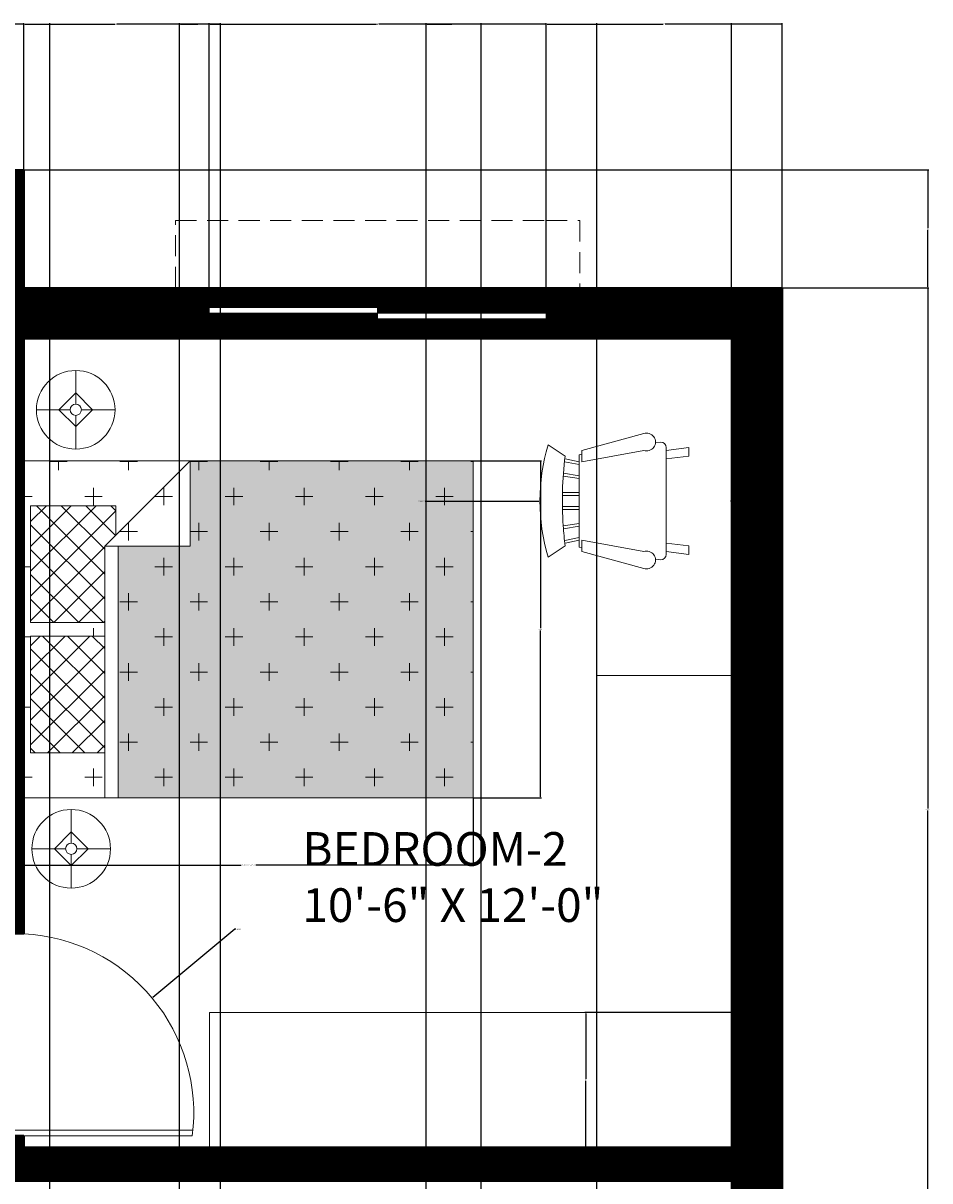
# Model space of a CAD drawing. Units: inches. Extents: x 557 to 1007, y 390 to 953.
# Tile 10 of 10: x 845 to 1007, y 747 to 953. Entities that reach past the tile are written whole.
import ezdxf

# ---------------------------------------------------------------- set-up
doc = ezdxf.new("R2010")
doc.units = ezdxf.units.IN
doc.header["$LTSCALE"] = 5
doc.header["$MEASUREMENT"] = 0
doc.linetypes.add('HIDDEN', pattern=[0.375, 0.25, -0.125])
for name, color, linetype, lineweight in [('A-ANNO-DIMS', 2, 'Continuous', 18), ('A-AREA-IDEN', 7, 'Continuous', 18), ('A-DOOR', 3, 'Continuous', 18), ('A-FLOR-CASE', 8, 'Continuous', 18), ('A-FURN', 8, 'Continuous', 18), ('A-FURN-PATT', 9, 'Continuous', 9), ('A-GLAZ', 4, 'Continuous', 18), ('A-GLAZ-OVHD', 8, 'HIDDEN', 13), ('A-WALL', 7, 'Continuous', 35), ('E-LITE', 2, 'Continuous', 13)]:
    doc.layers.add(name, color=color, linetype=linetype, lineweight=lineweight)
doc.layers.add('A-GLAZ-PATT', color=141, linetype='Continuous', lineweight=9, true_color=0xadddf7)
doc.layers.add('A-WALL-PATT', color=251, linetype='Continuous', lineweight=9, true_color=0x636466)
doc.styles.get("Standard").update_dxf_attribs({"font": 'arial.ttf'})
doc.dimstyles.get("Standard").update_dxf_attribs({"dimtxt": 0.18, "dimasz": 0.18, "dimexe": 0.18, "dimexo": 0.0625, "dimgap": 0.09, "dimtad": 0, "dimtih": 1, "dimtoh": 1, "dimdec": 4, "dimzin": 0, "dimdsep": 46, "dimtxsty": 'Standard', "dimcen": 0.09, "dimadec": 0, "dimazin": 0, "dimtfac": 1, "dimtdec": 4, "dimtofl": 0, "dimtmove": 0, "dimatfit": 3, "dimfxl": 1, "dimtolj": 1, "dimtzin": 0, "dimarcsym": 0})

# ---------------------------------------------------------------- blocks, each defined once
blk = doc.blocks.new('Chair - Rocking')
for p, q in [((-8, -4.5), (-10, -1.5)), ((8, -4.5), (10, -1.5)), ((-1.5, -4.05012), (-1.5, -7)), ((-1, -7), (-1, -4.05012)), ((1, -7), (1, -4.04655)), ((1.5, -4.05012), (1.5, -7)), ((-7.5, -4.5), (-7, -7)), ((-6.5, -7), (-7.02225, -4.43)), ((-4.5, -7), (-4.96674, -4.19951)), ((-4, -7), (-4.40532, -4.16272)), ((4, -7), (4.40187, -4.18694)), ((4.5, -7), (4.96761, -4.19437)), ((6.5, -7), (7, -4.4057)), ((7.5, -4.5), (7, -7)), ((-9, -7.5), (-12, -18.49999)), ((-7, -7.5), (-9, -7.5)), ((-9, -18.49999), (-7, -7.5)), ((-8.23428, -6.99939), (-8.3093, -7.47958)), ((-8.23041, -7), (8.23915, -7)), ((7, -7.5), (9, -7.5)), ((9, -18.49999), (7, -7.5)), ((8.31071, -7.48854), (8.23449, -7.00073)), ((9, -7.5), (12, -18.49999)), ((10.5, -21.49999), (10.3575, -20.58798)), ((-10.36644, -20.64523), (-10.5, -21.49999)), ((-9, -22.49999), (-9.5, -26.49999)), ((0, -22.49999), (-9.5, -22.49999)), ((-8, -26.49999), (-7.5, -22.49999)), ((0, -22.49999), (9.5, -22.49999)), ((8, -26.49999), (7.5, -22.49999)), ((9, -22.49999), (9.5, -26.49999)), ((-9.5, -26.49999), (-8, -26.49999)), ((9.5, -26.49999), (8, -26.49999))]:
    blk.add_line(p, q)
for centre, radius, start, end in [((0, -34.08333), 34.08333, 72.93847, 107.0615), ((0, -68.25004), 64.25, 82.84733, 93.92211), ((0, -68.25004), 64.25, 93.92211, 97.15267), ((-10.5, -18.99999), 1.58114, 161.5651, 18.43495), ((10.5, -18.99999), 1.58114, 161.5651, 18.43495), ((-9.5, -21.49999), 1, 180, 270), ((9.5, -21.49999), 1, 270, 0)]:
    blk.add_arc(centre, radius, start, end)
blk = doc.blocks.new('Lamp - Table')
for p, q in [((0, 7), (0, 1)), ((0, 3), (-3, 0)), ((3, 0), (0, 3)), ((-1, 0), (-7, 0)), ((-3, 0), (0, -3)), ((0, -3), (3, 0)), ((1, 0), (7, 0)), ((0, -1), (0, -7))]:
    blk.add_line(p, q)
for radius in [7, 1]:
    blk.add_circle((0, 0), radius)
blk = doc.blocks.new('BED-QUEEN-60x80-PLAN')
for p, q in [((0, 0), (0, 60)), ((0, 60), (80, 60)), ((29.6, 60), (14.4, 44.8)), ((29.6, 44.8), (29.6, 60)), ((80, 60), (80, 0)), ((1.2, 52), (16.4, 52)), ((1.2, 31.2), (1.2, 52)), ((16.4, 52), (16.4, 46.8)), ((14.4, 0), (14.4, 44.8)), ((14.4, 44.8), (29.6, 44.8)), ((16.8, 44.8), (16.8, 0)), ((14.4, 31.2), (1.2, 31.2)), ((1.2, 28.8), (14.4, 28.8)), ((1.2, 8), (1.2, 28.8)), ((14.4, 8), (1.2, 8)), ((80, 0), (0, 0))]:
    blk.add_line(p, q)
blk = doc.blocks.new('*D19')
at = {"layer": 'A-ANNO-DIMS', "color": 0, "lineweight": -2, "ltscale": 5, "transparency": 16777216}
for p, q in [((845.41, 815.04), (845.41, 802.92)), ((925.41, 815.04), (925.41, 802.92)), ((845.59, 803.1), (884.1, 803.1)), ((925.23, 803.1), (886.71, 803.1))]:
    blk.add_line(p, q, dxfattribs=at)
at = {"layer": 'A-ANNO-DIMS', "color": 0, "ltscale": 5, "transparency": 16777216}
for points in [[(845.59, 803.13), (845.59, 803.07), (845.41, 803.1)], [(925.23, 803.13), (925.23, 803.07), (925.41, 803.1)]]:
    blk.add_solid(points, dxfattribs=at)
at = {"layer": 'Defpoints', "color": 0, "ltscale": 5, "transparency": 16777216}
for p in [(845.41, 815.1), (925.41, 815.1), (925.41, 803.1)]:
    blk.add_point(p, dxfattribs=at)
at = {"layer": 'A-ANNO-DIMS', "color": 0, "ltscale": 5, "transparency": 16777216, "insert": (885.41, 803.1), "char_height": 0.18, "attachment_point": 5}
blk.add_mtext('\\A1;QUEEN BED 80 TYP.', dxfattribs=at)
blk = doc.blocks.new('*D20')
at = {"layer": 'A-ANNO-DIMS', "color": 0, "lineweight": -2, "ltscale": 5, "transparency": 16777216}
for p, q in [((925.47, 875.1), (937.59, 875.1)), ((937.41, 874.92), (937.41, 845.29)), ((937.41, 815.28), (937.41, 844.92)), ((925.47, 815.1), (937.59, 815.1))]:
    blk.add_line(p, q, dxfattribs=at)
at = {"layer": 'A-ANNO-DIMS', "color": 0, "ltscale": 5, "transparency": 16777216}
for points in [[(937.38, 874.92), (937.44, 874.92), (937.41, 875.1)], [(937.38, 815.28), (937.44, 815.28), (937.41, 815.1)]]:
    blk.add_solid(points, dxfattribs=at)
at = {"layer": 'Defpoints', "color": 0, "ltscale": 5, "transparency": 16777216}
for p in [(925.41, 875.1), (937.41, 875.1), (925.41, 815.1)]:
    blk.add_point(p, dxfattribs=at)
at = {"layer": 'A-ANNO-DIMS', "color": 0, "ltscale": 5, "transparency": 16777216, "insert": (937.41, 845.1), "char_height": 0.18, "attachment_point": 5}
blk.add_mtext('\\A1;60 TYP.', dxfattribs=at)
blk = doc.blocks.new('*D50')
at = {"layer": 'A-ANNO-DIMS', "color": 0, "lineweight": -2, "ltscale": 5, "transparency": 16777216}
for p, q in [((761.41, 926.97), (761.41, 953.03)), ((761.59, 952.85), (803.19, 952.85)), ((845.23, 952.85), (803.62, 952.85)), ((845.41, 926.97), (845.41, 953.03))]:
    blk.add_line(p, q, dxfattribs=at)
at = {"layer": 'A-ANNO-DIMS', "color": 0, "ltscale": 5, "transparency": 16777216}
for points in [[(761.59, 952.88), (761.59, 952.82), (761.41, 952.85)], [(845.23, 952.88), (845.23, 952.82), (845.41, 952.85)]]:
    blk.add_solid(points, dxfattribs=at)
at = {"layer": 'Defpoints', "color": 0, "ltscale": 5, "transparency": 16777216}
for p in [(845.41, 952.85), (761.41, 926.9), (845.41, 926.9)]:
    blk.add_point(p, dxfattribs=at)
at = {"layer": 'A-ANNO-DIMS', "color": 0, "ltscale": 5, "transparency": 16777216, "insert": (803.41, 952.85), "char_height": 0.18, "attachment_point": 5}
blk.add_mtext('\\A1;84', dxfattribs=at)
blk = doc.blocks.new('*D51')
at = {"layer": 'A-ANNO-DIMS', "color": 0, "lineweight": -2, "ltscale": 5, "transparency": 16777216}
for p, q in [((845.41, 905.97), (845.41, 953.03)), ((845.59, 952.85), (861.69, 952.85)), ((878.23, 952.85), (862.12, 952.85)), ((878.41, 905.97), (878.41, 953.03))]:
    blk.add_line(p, q, dxfattribs=at)
at = {"layer": 'A-ANNO-DIMS', "color": 0, "ltscale": 5, "transparency": 16777216}
for points in [[(845.59, 952.88), (845.59, 952.82), (845.41, 952.85)], [(878.23, 952.88), (878.23, 952.82), (878.41, 952.85)]]:
    blk.add_solid(points, dxfattribs=at)
at = {"layer": 'Defpoints', "color": 0, "ltscale": 5, "transparency": 16777216}
for p in [(878.41, 952.85), (845.41, 905.9), (878.41, 905.9)]:
    blk.add_point(p, dxfattribs=at)
at = {"layer": 'A-ANNO-DIMS', "color": 0, "ltscale": 5, "transparency": 16777216, "insert": (861.91, 952.85), "char_height": 0.18, "attachment_point": 5}
blk.add_mtext('\\A1;33', dxfattribs=at)
blk = doc.blocks.new('*D52')
at = {"layer": 'A-ANNO-DIMS', "color": 0, "lineweight": -2, "ltscale": 5, "transparency": 16777216}
for p, q in [((878.41, 905.97), (878.41, 953.03)), ((878.59, 952.85), (908.19, 952.85)), ((938.23, 952.85), (908.62, 952.85)), ((938.41, 905.97), (938.41, 953.03))]:
    blk.add_line(p, q, dxfattribs=at)
at = {"layer": 'A-ANNO-DIMS', "color": 0, "ltscale": 5, "transparency": 16777216}
for points in [[(878.59, 952.88), (878.59, 952.82), (878.41, 952.85)], [(938.23, 952.88), (938.23, 952.82), (938.41, 952.85)]]:
    blk.add_solid(points, dxfattribs=at)
at = {"layer": 'Defpoints', "color": 0, "ltscale": 5, "transparency": 16777216}
for p in [(938.41, 952.85), (878.41, 905.9), (938.41, 905.9)]:
    blk.add_point(p, dxfattribs=at)
at = {"layer": 'A-ANNO-DIMS', "color": 0, "ltscale": 5, "transparency": 16777216, "insert": (908.41, 952.85), "char_height": 0.18, "attachment_point": 5}
blk.add_mtext('\\A1;60', dxfattribs=at)
blk = doc.blocks.new('*D53')
at = {"layer": 'A-ANNO-DIMS', "color": 0, "lineweight": -2, "ltscale": 5, "transparency": 16777216}
for p, q in [((938.41, 905.97), (938.41, 953.03)), ((938.59, 952.85), (959.18, 952.85)), ((980.23, 952.85), (959.63, 952.85)), ((980.41, 905.97), (980.41, 953.03))]:
    blk.add_line(p, q, dxfattribs=at)
at = {"layer": 'A-ANNO-DIMS', "color": 0, "ltscale": 5, "transparency": 16777216}
for points in [[(938.59, 952.88), (938.59, 952.82), (938.41, 952.85)], [(980.23, 952.88), (980.23, 952.82), (980.41, 952.85)]]:
    blk.add_solid(points, dxfattribs=at)
at = {"layer": 'Defpoints', "color": 0, "ltscale": 5, "transparency": 16777216}
for p in [(980.41, 952.85), (938.41, 905.9), (980.41, 905.9)]:
    blk.add_point(p, dxfattribs=at)
at = {"layer": 'A-ANNO-DIMS', "color": 0, "ltscale": 5, "transparency": 16777216, "insert": (959.41, 952.85), "char_height": 0.18, "attachment_point": 5}
blk.add_mtext('\\A1;42', dxfattribs=at)
blk = doc.blocks.new('*D57')
at = {"layer": 'A-ANNO-DIMS', "color": 0, "lineweight": -2, "ltscale": 5, "transparency": 16777216}
for p, q in [((980.47, 905.9), (1006.54, 905.9)), ((1006.36, 905.72), (1006.36, 813.22)), ((1006.36, 720.36), (1006.36, 812.86)), ((980.47, 720.18), (1006.54, 720.18))]:
    blk.add_line(p, q, dxfattribs=at)
at = {"layer": 'A-ANNO-DIMS', "color": 0, "ltscale": 5, "transparency": 16777216}
for points in [[(1006.33, 905.72), (1006.39, 905.72), (1006.36, 905.9)], [(1006.33, 720.36), (1006.39, 720.36), (1006.36, 720.18)]]:
    blk.add_solid(points, dxfattribs=at)
at = {"layer": 'Defpoints', "color": 0, "ltscale": 5, "transparency": 16777216}
for p in [(980.41, 905.9), (1006.36, 905.9), (980.41, 720.18)]:
    blk.add_point(p, dxfattribs=at)
at = {"layer": 'A-ANNO-DIMS', "color": 0, "ltscale": 5, "transparency": 16777216, "insert": (1006.36, 813.04), "char_height": 0.18, "attachment_point": 5}
blk.add_mtext('\\A1;185.73', dxfattribs=at)
blk = doc.blocks.new('*D58')
at = {"layer": 'A-ANNO-DIMS', "color": 0, "lineweight": -2, "ltscale": 5, "transparency": 16777216}
for p, q in [((845.47, 926.9), (1006.54, 926.9)), ((1006.36, 926.72), (1006.36, 916.58)), ((1006.36, 906.08), (1006.36, 916.22)), ((980.47, 905.9), (1006.54, 905.9))]:
    blk.add_line(p, q, dxfattribs=at)
at = {"layer": 'A-ANNO-DIMS', "color": 0, "ltscale": 5, "transparency": 16777216}
for points in [[(1006.33, 926.72), (1006.39, 926.72), (1006.36, 926.9)], [(1006.33, 906.08), (1006.39, 906.08), (1006.36, 905.9)]]:
    blk.add_solid(points, dxfattribs=at)
at = {"layer": 'Defpoints', "color": 0, "ltscale": 5, "transparency": 16777216}
for p in [(845.41, 926.9), (1006.36, 926.9), (980.41, 905.9)]:
    blk.add_point(p, dxfattribs=at)
at = {"layer": 'A-ANNO-DIMS', "color": 0, "ltscale": 5, "transparency": 16777216, "insert": (1006.36, 916.4), "char_height": 0.18, "attachment_point": 5}
blk.add_mtext('\\A1;21', dxfattribs=at)
blk = doc.blocks.new('*D82')
at = {"layer": 'A-ANNO-DIMS', "color": 0, "lineweight": -2, "ltscale": 5, "transparency": 16777216}
for p, q in [((850.01, 665.94), (850.01, 953.03)), ((850.19, 952.85), (861.18, 952.85)), ((872.97, 952.85), (861.98, 952.85)), ((873.15, 661.94), (873.15, 953.03))]:
    blk.add_line(p, q, dxfattribs=at)
at = {"layer": 'A-ANNO-DIMS', "color": 0, "ltscale": 5, "transparency": 16777216}
for points in [[(850.19, 952.88), (850.19, 952.82), (850.01, 952.85)], [(872.97, 952.88), (872.97, 952.82), (873.15, 952.85)]]:
    blk.add_solid(points, dxfattribs=at)
at = {"layer": 'Defpoints', "color": 0, "ltscale": 5, "transparency": 16777216}
for p in [(873.15, 952.85), (850.01, 665.88), (873.15, 661.88)]:
    blk.add_point(p, dxfattribs=at)
at = {"layer": 'A-ANNO-DIMS', "color": 0, "ltscale": 5, "transparency": 16777216, "insert": (861.58, 952.85), "char_height": 0.18, "attachment_point": 5}
blk.add_mtext('\\A1;23.13', dxfattribs=at)
blk = doc.blocks.new('*D86')
at = {"layer": 'A-ANNO-DIMS', "color": 0, "lineweight": -2, "ltscale": 5, "transparency": 16777216}
for p, q in [((873.15, 661.94), (873.15, 953.03)), ((873.33, 952.85), (876.4, 952.85)), ((880.27, 952.85), (877.19, 952.85)), ((880.45, 663.9), (880.45, 953.03))]:
    blk.add_line(p, q, dxfattribs=at)
at = {"layer": 'A-ANNO-DIMS', "color": 0, "ltscale": 5, "transparency": 16777216}
for points in [[(873.33, 952.88), (873.33, 952.82), (873.15, 952.85)], [(880.27, 952.88), (880.27, 952.82), (880.45, 952.85)]]:
    blk.add_solid(points, dxfattribs=at)
at = {"layer": 'Defpoints', "color": 0, "ltscale": 5, "transparency": 16777216}
for p in [(880.45, 952.85), (880.45, 663.84), (873.15, 661.88)]:
    blk.add_point(p, dxfattribs=at)
at = {"layer": 'A-ANNO-DIMS', "color": 0, "ltscale": 5, "transparency": 16777216, "insert": (876.8, 952.85), "char_height": 0.18, "attachment_point": 5}
blk.add_mtext('\\A1;7.303', dxfattribs=at)
blk = doc.blocks.new('*D87')
at = {"layer": 'A-ANNO-DIMS', "color": 0, "lineweight": -2, "ltscale": 5, "transparency": 16777216}
for p, q in [((917.05, 663.9), (917.05, 953.03)), ((917.23, 952.85), (921.61, 952.85)), ((926.63, 952.85), (922.26, 952.85)), ((926.81, 662.58), (926.81, 953.03))]:
    blk.add_line(p, q, dxfattribs=at)
at = {"layer": 'A-ANNO-DIMS', "color": 0, "ltscale": 5, "transparency": 16777216}
for points in [[(917.23, 952.88), (917.23, 952.82), (917.05, 952.85)], [(926.63, 952.88), (926.63, 952.82), (926.81, 952.85)]]:
    blk.add_solid(points, dxfattribs=at)
at = {"layer": 'Defpoints', "color": 0, "ltscale": 5, "transparency": 16777216}
for p in [(926.81, 952.85), (917.05, 663.84), (926.81, 662.52)]:
    blk.add_point(p, dxfattribs=at)
at = {"layer": 'A-ANNO-DIMS', "color": 0, "ltscale": 5, "transparency": 16777216, "insert": (921.93, 952.85), "char_height": 0.18, "attachment_point": 5}
blk.add_mtext('\\A1;9.76', dxfattribs=at)
blk = doc.blocks.new('*D96')
at = {"layer": 'A-ANNO-DIMS', "color": 0, "lineweight": -2, "ltscale": 5, "transparency": 16777216}
for p, q in [((947.41, 536.97), (947.41, 953.03)), ((947.59, 952.85), (959.19, 952.85)), ((971.23, 952.85), (959.63, 952.85)), ((971.41, 512.97), (971.41, 953.03))]:
    blk.add_line(p, q, dxfattribs=at)
at = {"layer": 'A-ANNO-DIMS', "color": 0, "ltscale": 5, "transparency": 16777216}
for points in [[(947.59, 952.88), (947.59, 952.82), (947.41, 952.85)], [(971.23, 952.88), (971.23, 952.82), (971.41, 952.85)]]:
    blk.add_solid(points, dxfattribs=at)
at = {"layer": 'Defpoints', "color": 0, "ltscale": 5, "transparency": 16777216}
for p in [(971.41, 952.85), (947.41, 536.9), (971.41, 512.9)]:
    blk.add_point(p, dxfattribs=at)
at = {"layer": 'A-ANNO-DIMS', "color": 0, "ltscale": 5, "transparency": 16777216, "insert": (959.41, 952.85), "char_height": 0.18, "attachment_point": 5}
blk.add_mtext('\\A1;24', dxfattribs=at)
blk = doc.blocks.new('*D97')
at = {"layer": 'A-ANNO-DIMS', "color": 0, "lineweight": -2, "ltscale": 5, "transparency": 16777216}
for p, q in [((971.34, 776.9), (945.28, 776.9)), ((945.46, 776.72), (945.46, 765.08)), ((945.46, 753.08), (945.46, 764.72)), ((971.34, 752.9), (945.28, 752.9))]:
    blk.add_line(p, q, dxfattribs=at)
at = {"layer": 'A-ANNO-DIMS', "color": 0, "ltscale": 5, "transparency": 16777216}
for points in [[(945.43, 776.72), (945.49, 776.72), (945.46, 776.9)], [(945.43, 753.08), (945.49, 753.08), (945.46, 752.9)]]:
    blk.add_solid(points, dxfattribs=at)
at = {"layer": 'Defpoints', "color": 0, "ltscale": 5, "transparency": 16777216}
for p in [(945.46, 776.9), (971.41, 776.9), (971.41, 752.9)]:
    blk.add_point(p, dxfattribs=at)
at = {"layer": 'A-ANNO-DIMS', "color": 0, "ltscale": 5, "transparency": 16777216, "insert": (945.46, 764.9), "char_height": 0.18, "attachment_point": 5}
blk.add_mtext('\\A1;24', dxfattribs=at)
blk = doc.blocks.new('*D108')
at = {"layer": 'A-ANNO-DIMS', "color": 0, "lineweight": -2, "ltscale": 5, "transparency": 16777216}
for p, q in [((882.99, 791.73), (868.4, 779.57)), ((883.17, 791.73), (882.99, 791.73)), ((843.63, 759), (843.81, 759)), ((843.72, 758.91), (843.72, 759.09))]:
    blk.add_line(p, q, dxfattribs=at)
at = {"layer": 'A-ANNO-DIMS', "color": 0, "ltscale": 5, "transparency": 16777216}
blk.add_solid([(868.38, 779.59), (868.42, 779.55), (868.26, 779.45)], dxfattribs=at)
at = {"layer": 'Defpoints', "color": 0, "ltscale": 5, "transparency": 16777216}
for p in [(868.26, 779.45), (843.72, 759)]:
    blk.add_point(p, dxfattribs=at)
at = {"layer": 'A-ANNO-DIMS', "color": 0, "ltscale": 5, "transparency": 16777216, "insert": (883.65, 791.73), "char_height": 0.18, "attachment_point": 5}
blk.add_mtext('\\A1;R31.95', dxfattribs=at)
blk = doc.blocks.new('*D113')
at = {"layer": 'A-ANNO-DIMS', "color": 0, "lineweight": -2, "ltscale": 5, "transparency": 16777216}
for p, q in [((916.84, 867.95), (937.11, 867.95)), ((971.29, 867.96), (971.47, 867.96)), ((971.38, 867.87), (971.38, 868.05))]:
    blk.add_line(p, q, dxfattribs=at)
at = {"layer": 'A-ANNO-DIMS', "color": 0, "ltscale": 5, "transparency": 16777216}
blk.add_solid([(937.11, 867.98), (937.11, 867.92), (937.29, 867.95)], dxfattribs=at)
at = {"layer": 'Defpoints', "color": 0, "ltscale": 5, "transparency": 16777216}
for p in [(937.29, 867.95), (971.38, 867.96)]:
    blk.add_point(p, dxfattribs=at)
at = {"layer": 'A-ANNO-DIMS', "color": 0, "ltscale": 5, "transparency": 16777216, "insert": (916.17, 867.95), "char_height": 0.18, "attachment_point": 5}
blk.add_mtext('\\A1;3X R34.08', dxfattribs=at)

msp = doc.modelspace()

# ---------------------------------------------------------------- hatches: boundary and pattern name
at = {"layer": 'A-FURN-PATT', "ltscale": 5}
h = msp.add_hatch(dxfattribs=at)
h.set_pattern_fill('GRAVEL', color=256, scale=25)
h.set_pattern_definition([(228.01279, (18, 25), (-200, -225), [3.3634, -332.9772]), (184.96974, (15.75, 22.5), (300, 25), [5.7717, -571.39812]), (132.51045, (10, 22), (250, -275), [4.0697, -402.9008]), (267.27369, (0.25, 15.75), (25, 500), [5.25595, -520.33895]), (292.83365, (0, 10.5), (-125, 300), [5.15387, -510.23433]), (357.27369, (2, 5.75), (-500, 25), [5.25595, -520.33895]), (37.69424, (7.25, 5.5), (-325, -250), [6.95072, -688.1212]), (72.25533, (12.75, 9.75), (175, 550), [6.5622, -649.65804]), (121.42957, (14.75, 16), (-200, 325), [5.27375, -522.10183]), (175.23636, (12, 20.5), (275, -25), [6.0208, -295.01906]), (222.39744, (6, 21), (-300, -275), [7.7862, -770.83438]), (138.81407, (25, 15.5), (-175, 150), [2.65752, -263.0961]), (171.46923, (23, 17.25), (325, -50), [5.05593, -500.5378]), (225, (18, 18), (-3e-15, -25), [3.53552, -31.8198]), (203.1986, (16.25, 21), (125, 50), [1.90395, -188.49038]), (291.8014, (14.5, 20.25), (-25, 75), [2.69257, -131.93655]), (30.96376, (15.5, 17.75), (75, 50), [4.37322, -141.40057]), (161.56505, (19.25, 20), (50, -25), [3.16228, -75.89467]), (16.38954, (0, 20.25), (250, 75), [4.43, -438.57113]), (70.34618, (4.25, 21.5), (-100, -275), [3.71652, -367.9352]), (293.1986, (19.25, 25), (-50, 125), [3.80788, -186.58645]), (343.61046, (20.75, 21.5), (-250, 75), [4.43, -438.57113]), (339.44395, (0, 4.75), (-125, 50), [4.272, -209.3281]), (294.77514, (4, 3.25), (-125, 275), [3.57945, -354.36608]), (66.8014, (19.5, 0), (50, 125), [3.80788, -186.58645]), (17.35402, (21, 3.5), (-325, -100), [4.19078, -414.8856]), (69.44395, (7.25, 0), (-50, -125), [2.136, -211.4641]), (101.30993, (18, 0), (-25, 100), [1.27475, -126.20074]), (165.96376, (17.75, 1.25), (75, -25), [5.15388, -97.92377]), (186.00901, (12.75, 2.5), (250, 25), [4.77625, -472.84808]), (303.69007, (15.5, 15.5), (-25, 50), [3.60555, -86.53323]), (353.15723, (17.5, 12.5), (425, -50), [6.29485, -623.18907]), (60.9454, (23.75, 11.75), (-100, -175), [2.5739, -254.81685]), (90, (25, 14), (-25, 25), [1.5, -23.5]), (120.25644, (12.25, 3.25), (100, -175), [3.4731, -343.838]), (48.01279, (10.5, 6.25), (200, 225), [6.7268, -329.6138]), (0, (15, 11.25), (25, 25), [6.5, -18.5]), (325.30485, (21.5, 11.25), (250, -175), [3.95285, -391.33186]), (254.0546, (24.75, 9), (-25, -100), [3.64005, -178.3627]), (207.64598, (23.75, 5.5), (-475, -250), [5.92662, -586.73685]), (175.42608, (18.5, 2.75), (-325, 25), [6.26997, -620.72684])])
h.paths.add_polyline_path([(615.2525, 688.5, 1), (640.7475, 688.5, 1)])
h.paths.add_polyline_path([(917.0544, 663.8414, 0.33333323), (915.2241, 665.6717), (882.2793, 665.6717, 0.33333323), (880.449, 663.8414), (880.449, 649.1992, 0.33333323), (882.2793, 647.369), (915.2241, 647.369, 0.33333323), (917.0544, 649.1992)])
h.paths.add_polyline_path([(828.0807, 699.7098), (756.0807, 699.7098), (756.0807, 663.7098), (828.0807, 663.7098)])
h.paths.add_polyline_path([(787.5651, 663.7098), (768.5964, 663.7098), (769.8463, 655.7098), (786.3151, 655.7098)])
h.paths.add_polyline_path([(815.5651, 663.7098), (796.5964, 663.7098), (797.8463, 655.7098), (814.3151, 655.7098)])
h.paths.add_polyline_path([(836.0807, 689.9442), (828.0807, 691.1942), (828.0807, 672.2255), (836.0807, 673.4755)])
h.paths.add_polyline_path([(756.0807, 691.1942), (748.0807, 689.9442), (748.0807, 673.4755), (756.0807, 672.2255)])
h.paths.add_polyline_path([(786.3151, 707.7098), (769.8463, 707.7098), (768.5964, 699.7098), (787.5651, 699.7098)])
h.paths.add_polyline_path([(814.3151, 707.7098), (797.8463, 707.7098), (796.5964, 699.7098), (815.5651, 699.7098)])
h.paths.add_polyline_path([(917.4362, 607.3575), (889.5896, 607.3575), (889.5896, 586.4726), (917.4362, 586.4726)])
h.paths.add_polyline_path([(721.4053, 881.8539), (671.0053, 881.8539), (671.0053, 866.6539), (658.2053, 866.6539), (658.2053, 821.8539), (721.4053, 821.8539)])
h.paths.add_polyline_path([(925.4053, 875.1046), (875.0053, 875.1046), (875.0053, 859.9046), (862.2053, 859.9046), (862.2053, 815.1046), (925.4053, 815.1046)])
h.paths.add_polyline_path([(721.4053, 558.9046), (671.0053, 558.9046), (671.0053, 543.7046), (658.2053, 543.7046), (658.2053, 498.9046), (721.4053, 498.9046)])
at = {"layer": 'A-FURN-PATT'}
h = msp.add_hatch(dxfattribs=at)
h.set_pattern_fill('CROSS', color=256, scale=25)
h.paths.add_polyline_path([(925.4053, 875.1046), (875.0053, 875.1046), (875.0053, 859.9046), (862.2053, 859.9046), (862.2053, 815.1046), (925.4053, 815.1046)])
h.paths.add_polyline_path([(721.4053, 881.8539), (671.0053, 881.8539), (671.0053, 866.6539), (658.2053, 866.6539), (658.2053, 821.8539), (721.4053, 821.8539)])
h.paths.add_polyline_path([(671.0053, 881.8539), (655.8053, 866.6539), (671.0053, 866.6539)], flags=17)
h.paths.add_polyline_path([(671.0053, 881.8539), (641.4053, 881.8539), (641.4053, 821.8539), (655.8053, 821.8539), (655.8053, 829.8539), (642.6053, 829.8539), (642.6053, 850.6539), (655.8053, 850.6539), (655.8053, 853.0539), (642.6053, 853.0539), (642.6053, 873.8539), (657.8053, 873.8539), (657.8053, 868.6539)])
h.paths.add_polyline_path([(875.0053, 875.1046), (859.8053, 859.9046), (875.0053, 859.9046)], flags=17)
h.paths.add_polyline_path([(875.0053, 875.1046), (845.4053, 875.1046), (845.4053, 815.1046), (859.8053, 815.1046), (859.8053, 823.1046), (846.6053, 823.1046), (846.6053, 843.9046), (859.8053, 843.9046), (859.8053, 846.3046), (846.6053, 846.3046), (846.6053, 867.1046), (861.8053, 867.1046), (861.8053, 861.9046)])
h.paths.add_polyline_path([(721.4053, 558.9046), (671.0053, 558.9046), (671.0053, 543.7046), (658.2053, 543.7046), (658.2053, 498.9046), (721.4053, 498.9046)])
h.paths.add_polyline_path([(671.0053, 558.9046), (641.4053, 558.9046), (641.4053, 498.9046), (655.8053, 498.9046), (655.8053, 506.9046), (642.6053, 506.9046), (642.6053, 527.7046), (655.8053, 527.7046), (655.8053, 530.1046), (642.6053, 530.1046), (642.6053, 550.9046), (657.8053, 550.9046), (657.8053, 545.7046)])
h.paths.add_polyline_path([(671.0053, 558.9046), (657.8053, 545.7046), (655.8053, 543.7046), (671.0053, 543.7046)], flags=17)
h.paths.add_polyline_path([(873.1461, 661.8773, 0.41421356), (868.1461, 666.8773, -0.12244426), (867.1516, 666.8773), (855.014, 666.8773), (855.014, 647.2429), (867.4581, 647.2429, -0.08537395), (868.1461, 647.2429, 0.41421356), (873.1461, 652.2429)])
h.paths.add_polyline_path([(917.0544, 663.8414, 0.33333323), (915.2241, 665.6717), (882.2793, 665.6717, 0.33333323), (880.449, 663.8414), (880.449, 649.1992, 0.33333323), (882.2793, 647.369), (915.2241, 647.369, 0.33333323), (917.0544, 649.1992)])
h.paths.add_polyline_path([(944.9465, 667.5202), (932.6561, 667.5202, -0.10407786), (931.8144, 667.5202, 0.41421356), (926.8144, 662.5202), (926.8144, 652.8858, 0.41421356), (931.8144, 647.8858, -0.05611627), (932.2647, 647.8858), (944.9465, 647.8858)])
h.paths.add_polyline_path([(928.8341, 635.542, 0.41421356), (923.8341, 640.542), (914.1997, 640.542, 0.41421356), (909.1997, 635.542), (909.1997, 622.4099), (923.8341, 622.4099, 0.41421356), (928.8341, 627.4099)])
h.paths.add_polyline_path([(909.1997, 635.542, 0.41421356), (904.1997, 640.542), (894.5653, 640.542, 0.41421356), (889.5653, 635.542), (889.5653, 622.4099), (909.1997, 622.4099)])
h.paths.add_polyline_path([(889.5653, 635.542, 0.41421356), (884.5653, 640.542), (874.9308, 640.542, 0.41421356), (869.9308, 635.542), (869.9308, 627.4099, 0.41421356), (874.9308, 622.4099), (889.5653, 622.4099)])
h = msp.add_hatch(dxfattribs=at)
h.set_pattern_fill('ANSI37', color=256, scale=25)
h.paths.add_polyline_path([(655.8053, 866.6539), (657.8053, 868.6539), (657.8053, 873.8539), (642.6053, 873.8539), (642.6053, 853.0539), (655.8053, 853.0539)])
h.paths.add_polyline_path([(655.8053, 850.6539), (642.6053, 850.6539), (642.6053, 829.8539), (655.8053, 829.8539)])
h.paths.add_polyline_path([(859.8053, 859.9046), (861.8053, 861.9046), (861.8053, 867.1046), (846.6053, 867.1046), (846.6053, 846.3046), (859.8053, 846.3046)])
h.paths.add_polyline_path([(859.8053, 843.9046), (846.6053, 843.9046), (846.6053, 823.1046), (859.8053, 823.1046)])
h.paths.add_polyline_path([(655.8053, 527.7046), (642.6053, 527.7046), (642.6053, 506.9046), (655.8053, 506.9046)])
h.paths.add_polyline_path([(657.8053, 545.7046), (657.8053, 550.9046), (642.6053, 550.9046), (642.6053, 530.1046), (655.8053, 530.1046), (655.8053, 543.7046)])
at = {"layer": 'A-GLAZ-PATT'}
h = msp.add_hatch(dxfattribs=at)
h.set_pattern_fill('ANSI31', color=256)
h.paths.add_polyline_path([(635.9053, 814.7688), (636.9053, 814.7688), (636.9053, 838.7688), (632.4053, 838.7688), (632.4053, 790.7688), (635.9053, 790.7688)])
h.paths.add_polyline_path([(641.4053, 838.7688), (637.9053, 838.7688), (637.9053, 814.7688), (636.9053, 814.7688), (636.9053, 790.7688), (641.4053, 790.7688)])
h.paths.add_polyline_path([(603.4053, 728.9046, -0.41421356), (623.4053, 748.9046), (632.4053, 748.9046), (632.4053, 752.9046), (623.4053, 752.9046, 0.41421356), (599.4053, 728.9046), (599.4053, 614.9046), (603.4053, 614.9046)])
h.paths.add_polyline_path([(632.4053, 743.9046), (632.4053, 747.9046), (623.4053, 747.9046, 0.41421356), (604.4053, 728.9046), (604.4053, 614.9046), (608.4053, 614.9046), (608.4053, 719.9046, -0.41421356)])
h.paths.add_polyline_path([(683.4053, 722.9046), (678.9053, 722.9046), (678.9053, 698.9046), (679.9053, 698.9046), (679.9053, 662.9046), (678.9053, 662.9046), (678.9053, 638.9046), (683.4053, 638.9046)])
h.paths.add_polyline_path([(678.9053, 698.9046), (677.9053, 698.9046), (677.9053, 722.9046), (674.4053, 722.9046), (674.4053, 638.9046), (677.9053, 638.9046), (677.9053, 662.9046), (678.9053, 662.9046)])
h.paths.add_polyline_path([(635.9053, 593.9046), (632.4053, 593.9046), (632.4053, 557.9046), (635.9053, 557.9046)])
h.paths.add_polyline_path([(641.4053, 593.9046), (637.9053, 593.9046), (637.9053, 557.9046), (641.4053, 557.9046)])
h.paths.add_polyline_path([(764.9579, 448.9046), (716.9579, 448.9046), (716.9579, 445.4046), (740.9579, 445.4046), (740.9579, 444.4046), (764.9579, 444.4046)])
h.paths.add_polyline_path([(764.9579, 443.4046), (740.9579, 443.4046), (740.9579, 444.4046), (716.9579, 444.4046), (716.9579, 439.9046), (764.9579, 439.9046)])
h.paths.add_polyline_path([(938.4053, 905.9046), (878.4053, 905.9046), (878.4053, 902.4046), (908.4053, 902.4046), (908.4053, 901.4046), (938.4053, 901.4046)])
h.paths.add_polyline_path([(938.4053, 900.4046), (908.4053, 900.4046), (908.4053, 901.4046), (878.4053, 901.4046), (878.4053, 896.9046), (938.4053, 896.9046)])
h.paths.add_polyline_path([(724.9087, 905.9046), (676.9087, 905.9046), (676.9087, 902.4046), (701.4053, 902.4046), (701.4053, 901.4046), (724.9087, 901.4046)])
h.paths.add_polyline_path([(724.9087, 900.4046), (701.4053, 900.4046), (701.4053, 901.4046), (676.9087, 901.4046), (676.9087, 896.9046), (724.9087, 896.9046)])
h.paths.add_polyline_path([(832.0625, 905.9046), (808.0625, 905.9046), (808.0625, 902.4046), (832.0625, 902.4046)])
h.paths.add_polyline_path([(832.0625, 900.4046), (808.0625, 900.4046), (808.0625, 896.9046), (832.0625, 896.9046)])
at = {"layer": 'A-WALL-PATT'}
h = msp.add_hatch(dxfattribs=at)
h.set_pattern_fill('ANSI31', color=256)
h.paths.add_polyline_path([(808.0625, 905.9046), (767.4053, 905.9046), (767.4053, 920.9046), (839.4053, 920.9046), (839.4053, 905.9046), (832.0625, 905.9046), (832.0625, 896.9046), (839.4053, 896.9046), (839.4053, 800.9046), (837.4053, 800.9046), (837.4053, 794.9046), (839.4053, 794.9046), (839.4053, 790.9046), (845.4053, 790.9046), (845.4053, 896.9046), (878.4053, 896.9046), (878.4053, 905.9046), (845.4053, 905.9046), (845.4053, 926.9046), (761.4053, 926.9046), (761.4053, 914.9046), (761.4053, 905.9046), (724.9087, 905.9046), (724.9087, 896.9046), (761.4053, 896.9046), (761.4053, 752.9046), (759.4053, 752.9046), (759.4053, 746.9046), (767.4053, 746.9046), (767.4053, 794.9046), (807.4053, 794.9046), (807.4053, 800.9046), (767.4053, 800.9046), (767.4053, 896.9046), (808.0625, 896.9046)])
h.paths.add_polyline_path([(676.9087, 905.9046), (632.4053, 905.9046), (632.4053, 838.7688), (641.4053, 838.7688), (641.4053, 881.8539), (641.4053, 896.9046), (676.9087, 896.9046)])
h.paths.add_polyline_path([(980.4053, 905.9046), (938.4053, 905.9046), (938.4053, 896.9046), (971.4053, 896.9046), (971.4053, 752.9046), (845.4053, 752.9046), (845.4053, 754.9046), (839.4053, 754.9046), (839.4053, 746.9046), (971.4053, 746.9046), (971.4053, 720.1788), (980.4053, 720.1788)])
h.paths.add_polyline_path([(723.4053, 752.9046), (641.4053, 752.9046), (641.4053, 790.7688), (632.4053, 790.7688), (632.4053, 743.9046), (674.4053, 743.9046), (674.4053, 722.9046), (683.4053, 722.9046), (683.4053, 746.9046), (723.4053, 746.9046)])
h.paths.add_polyline_path([(980.4053, 684.1788), (971.4053, 684.1788), (971.4053, 614.9046), (845.4053, 614.9046), (845.4053, 608.9046), (971.4053, 608.9046), (971.4053, 512.9046), (908.7697, 512.9046), (908.7697, 508.9046), (971.4053, 508.9046), (971.4053, 448.9046), (845.4053, 448.9046), (845.4053, 508.9046), (878.7697, 508.9046), (878.7697, 512.9046), (845.4053, 512.9046), (845.4053, 562.9046), (779.4053, 562.9046), (779.4053, 614.9046), (761.4053, 614.9046), (761.4053, 608.9046), (773.4053, 608.9046), (773.4053, 512.636), (779.4053, 512.636), (779.4053, 556.9046), (839.4053, 556.9046), (839.4053, 448.9046), (830.432, 448.9046), (830.432, 439.9046), (839.4053, 439.9046), (839.4053, 433.0506), (839.4053, 421.9046), (779.4053, 421.9046), (779.4053, 439.9046), (796.9656, 439.9046), (806.432, 439.9046), (806.432, 448.9046), (779.4053, 448.9046), (779.4053, 482.636), (773.4053, 482.636), (773.4053, 448.9046), (764.9579, 448.9046), (764.9579, 439.9046), (773.4053, 439.9046), (773.4053, 415.9046), (845.4053, 415.9046), (845.4053, 439.9046), (980.4053, 439.9046)])
h.paths.add_polyline_path([(716.9579, 448.9046), (641.4053, 448.9046), (641.4053, 557.9046), (632.4053, 557.9046), (632.4053, 439.9046), (716.9579, 439.9046)])
h.paths.add_polyline_path([(725.4053, 614.9046), (683.4053, 614.9046), (683.4053, 638.9046), (674.4053, 638.9046), (674.4053, 614.9046), (608.4053, 614.9046), (582.8236, 614.9046), (582.8236, 605.9046), (599.4053, 605.9046), (632.4053, 605.9046), (641.4053, 605.9046), (641.4053, 608.9046), (725.4053, 608.9046)])
h.paths.add_polyline_path([(641.4053, 605.9046), (632.4053, 605.9046), (632.4053, 593.9046), (641.4053, 593.9046)])

# ---------------------------------------------------------------- linework, layer by layer
at = {"layer": 'A-DOOR'}
for p, q in [((839.4053, 755.9046), (875.4053, 755.9046)), ((839.4053, 754.9046), (875.4053, 754.9046))]:
    msp.add_line(p, q, dxfattribs=at)
msp.add_arc((843.7185, 758.999), 31.9502, 352.637319, 86.973824, dxfattribs=at)
at = {"layer": 'A-FLOR-CASE'}
for p, q in [((947.4053, 896.9046), (947.4053, 836.9046)), ((947.4053, 836.9046), (971.4053, 836.9046)), ((878.4796, 776.9046), (971.4053, 776.9046)), ((878.4796, 752.9046), (878.4796, 776.9046))]:
    msp.add_line(p, q, dxfattribs=at)
at = {"layer": 'A-GLAZ'}
for p, q in [((878.4053, 896.9046), (878.4053, 905.9046)), ((938.4053, 896.9046), (938.4053, 905.9046)), ((908.4053, 902.4046), (878.4053, 902.4046)), ((938.4053, 901.4046), (878.4053, 901.4046)), ((908.4053, 900.4046), (908.4053, 902.4046)), ((938.4053, 900.4046), (908.4053, 900.4046))]:
    msp.add_line(p, q, dxfattribs=at)
at = {"layer": 'A-GLAZ-OVHD', "ltscale": 3}
for p, q in [((872.4053, 905.9046), (872.4053, 917.9046)), ((872.4053, 917.9046), (938.4053, 917.9046)), ((938.4053, 917.9046), (944.4053, 917.9046)), ((944.4053, 917.9046), (944.4053, 905.9046)), ((878.4053, 905.9046), (872.4053, 905.9046))]:
    msp.add_line(p, q, dxfattribs=at)
at = {"layer": 'A-WALL'}
for p, q in [((761.4053, 926.9046), (845.4053, 926.9046)), ((845.4053, 926.9046), (845.4053, 905.9046)), ((845.4053, 905.9046), (980.4053, 905.9046)), ((980.4053, 905.9046), (980.4053, 720.1788)), ((845.4053, 896.9046), (845.4053, 790.9046)), ((845.4053, 896.9046), (971.4053, 896.9046)), ((971.4053, 896.9046), (971.4053, 752.9046)), ((845.4053, 790.9046), (839.4053, 790.9046)), ((845.4053, 754.9046), (839.4053, 754.9046)), ((845.4053, 754.9046), (845.4053, 752.9046)), ((845.4053, 752.9046), (971.4053, 752.9046)), ((839.4053, 746.9046), (971.4053, 746.9046)), ((971.4053, 746.9046), (971.4053, 720.1788))]:
    msp.add_line(p, q, dxfattribs=at)

# ---------------------------------------------------------------- block references
at = {"layer": 'A-FURN', "rotation": 90}
msp.add_blockref('Chair - Rocking', (937.2918, 867.9551), dxfattribs=at)
at = {"layer": 'A-FURN'}
msp.add_blockref('BED-QUEEN-60x80-PLAN', (845.405, 815.105), dxfattribs=at)
at = {"layer": 'E-LITE', "rotation": 90}
for p in [(854.6469, 884.1888), (853.839, 806.0247)]:
    msp.add_blockref('Lamp - Table', p, dxfattribs=at)

# ---------------------------------------------------------------- texts
at = {"layer": 'A-AREA-IDEN', "insert": (895, 809), "char_height": 6, "attachment_point": 1}
msp.add_mtext_dynamic_manual_height_columns('BEDROOM-2\\P10\'-6" X 12\'-0"', width=125, gutter_width=1, heights=[0], dxfattribs=at)

# ---------------------------------------------------------------- dimensions: what is measured, and where the dimension line sits
at = {"layer": 'A-ANNO-DIMS', "ltscale": 5}
for base, p1, p2, override, picture, middle in [((845.4053, 952.8546), (761.4053, 926.9046), (845.4053, 926.9046), {"dimdec": 0, "dimlfac": 1, "dimrnd": 0, "dimzin": 0, "dimdsep": 46, "dimlunit": 2}, '*D50', (803.4053, 952.8546)), ((878.4053, 952.8546), (845.4053, 905.9046), (878.4053, 905.9046), {"dimdec": 0, "dimlfac": 1, "dimrnd": 0, "dimzin": 0, "dimdsep": 46, "dimlunit": 2}, '*D51', (861.9053, 952.8546)), ((873.1461, 952.8546), (850.014, 665.8773), (873.1461, 661.8773), {"dimdec": 2, "dimlfac": 1, "dimrnd": 0, "dimzin": 0, "dimdsep": 46, "dimlunit": 2}, '*D82', (861.58, 952.8546)), ((880.449, 952.8546), (873.1461, 661.8773), (880.449, 663.8414), {"dimdec": 3, "dimlfac": 1, "dimrnd": 0, "dimzin": 0, "dimdsep": 46, "dimlunit": 2}, '*D86', (876.7975, 952.8546)), ((938.4053, 952.8546), (878.4053, 905.9046), (938.4053, 905.9046), {"dimdec": 0, "dimlfac": 1, "dimrnd": 0, "dimzin": 0, "dimdsep": 46, "dimlunit": 2}, '*D52', (908.4053, 952.8546)), ((926.8144, 952.8546), (917.0544, 663.8414), (926.8144, 662.5202), {"dimdec": 2, "dimlfac": 1, "dimrnd": 0, "dimzin": 0, "dimdsep": 46, "dimlunit": 2}, '*D87', (921.9344, 952.8546)), ((980.4053, 952.8546), (938.4053, 905.9046), (980.4053, 905.9046), {"dimdec": 0, "dimlfac": 1, "dimrnd": 0, "dimzin": 0, "dimdsep": 46, "dimlunit": 2}, '*D53', (959.4053, 952.8546)), ((971.4053, 952.8546), (947.4053, 536.9046), (971.4053, 512.9046), {"dimdec": 0, "dimlfac": 1, "dimrnd": 0, "dimzin": 0, "dimdsep": 46, "dimlunit": 2}, '*D96', (959.4053, 952.8546))]:
    dim = msp.add_linear_dim(base=base, p1=p1, p2=p2, dimstyle='Standard', override=override, dxfattribs=at)
    dim.commit()
    dim.dimension.update_dxf_attribs({"geometry": picture, "text_midpoint": middle})
for base, p1, p2, override, picture, middle in [((1006.3553, 926.9046), (980.4053, 905.9046), (845.4053, 926.9046), {"dimdec": 0, "dimlfac": 1, "dimrnd": 0, "dimzin": 0, "dimdsep": 46, "dimlunit": 2}, '*D58', (1006.3553, 916.4046)), ((1006.3553, 905.9046), (980.4053, 720.1788), (980.4053, 905.9046), {"dimdec": 2, "dimlfac": 1, "dimrnd": 0, "dimzin": 0, "dimdsep": 46, "dimlunit": 2}, '*D57', (1006.3553, 813.0417)), ((945.4553, 776.9046), (971.4053, 752.9046), (971.4053, 776.9046), {"dimdec": 0, "dimlfac": 1, "dimrnd": 0, "dimzin": 0, "dimdsep": 46, "dimlunit": 2}, '*D97', (945.4553, 764.9046))]:
    dim = msp.add_linear_dim(base=base, p1=p1, p2=p2, angle=90, dimstyle='Standard', override=override, dxfattribs=at)
    dim.commit()
    dim.dimension.update_dxf_attribs({"geometry": picture, "text_midpoint": middle})
dim = msp.add_linear_dim(base=(937.4053, 875.1046), p1=(925.4053, 815.1046), p2=(925.4053, 875.1046), angle=90, text='<> TYP.', dimstyle='Standard', override={"dimdec": 0, "dimlfac": 1, "dimrnd": 0, "dimzin": 0, "dimdsep": 46, "dimlunit": 2}, dxfattribs=at)
dim.commit()
dim.dimension.update_dxf_attribs({"geometry": '*D20', "text_midpoint": (937.4053, 845.1046)})
dim = msp.add_radius_dim(center=(971.3751, 867.9551), mpoint=(937.2918, 867.955), text='3X <>', dimstyle='Standard', override={"dimdec": 2, "dimlfac": 1, "dimrnd": 0, "dimzin": 0, "dimdsep": 46, "dimlunit": 2}, dxfattribs=at)
dim.commit()
dim.dimension.update_dxf_attribs({"geometry": '*D113', "text_midpoint": (916.8418, 867.9549), "dimtype": 164})
dim = msp.add_linear_dim(base=(925.4053, 803.1046), p1=(845.4053, 815.1046), p2=(925.4053, 815.1046), text='QUEEN BED <> TYP.', dimstyle='Standard', override={"dimdec": 0, "dimlfac": 1, "dimrnd": 0, "dimzin": 0, "dimdsep": 46, "dimlunit": 2}, dxfattribs=at)
dim.commit()
dim.dimension.update_dxf_attribs({"geometry": '*D19', "text_midpoint": (885.4053, 803.1046)})
dim = msp.add_radius_dim(center=(843.7185, 758.999), mpoint=(868.2632, 779.4531), dimstyle='Standard', override={"dimdec": 2, "dimlfac": 1, "dimrnd": 0, "dimzin": 0, "dimdsep": 46, "dimlunit": 2}, dxfattribs=at)
dim.commit()
dim.dimension.update_dxf_attribs({"geometry": '*D108', "text_midpoint": (883.6505, 791.7256), "dimtype": 164})

doc.saveas('drawing.dxf')
